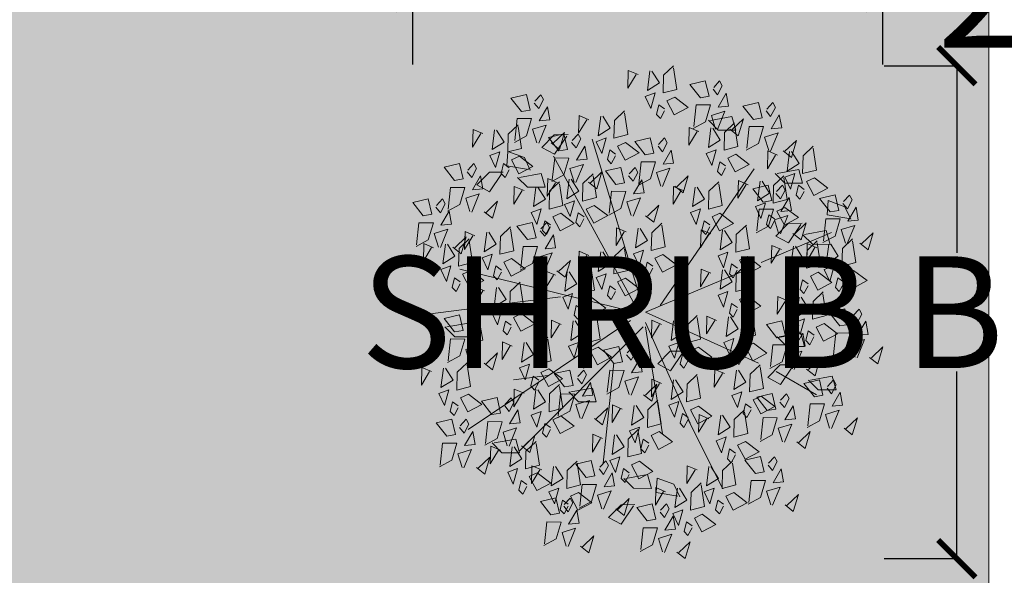
# Model space of a CAD drawing. Units: inches. Extents: x 1704 to 6393, y -157 to 1172.
# Tile 93 of 122: x 2667 to 2720, y 912 to 942. Entities that reach past the tile are written whole.
import ezdxf

# ---------------------------------------------------------------- set-up
doc = ezdxf.new("R2010")
doc.units = ezdxf.units.IN
doc.header["$MEASUREMENT"] = 0
for name, color, linetype, lineweight in [('A-ANNO-DIMS', 7, 'Continuous', 13), ('L-HRDS', 8, 'Continuous', 18), ('L-shrub', 74, 'Continuous', 18)]:
    doc.layers.add(name, color=color, linetype=linetype, lineweight=lineweight)
doc.layers.add('L-HRDS-PATT', color=9, linetype='Continuous', lineweight=13, true_color=0xc5c1ba)
doc.styles.get("Standard").update_dxf_attribs({"font": 'arial.ttf'})
doc.dimstyles.get("Standard").update_dxf_attribs({"dimtxt": 6, "dimasz": 2, "dimexe": 0.18, "dimexo": 0.0625, "dimgap": 0.09, "dimtad": 0, "dimtih": 1, "dimtoh": 1, "dimdec": 1, "dimzin": 0, "dimdsep": 46, "dimlunit": 3, "dimtxsty": 'Standard', "dimblk": 'ARCHTICK', "dimcen": 0.09, "dimadec": 0, "dimazin": 0, "dimtfac": 1, "dimtdec": 1, "dimtofl": 0, "dimtmove": 0, "dimatfit": 3, "dimfxl": 1, "dimtolj": 1, "dimtzin": 0, "dimarcsym": 0})

# ---------------------------------------------------------------- blocks, each defined once
blk = doc.blocks.new('flower shrub 2')
at = {"layer": 'L-shrub'}
for p, q in [((-106.2, 211.8), (-93, 218)), ((-112.6, 194.3), (-106.2, 211.8)), ((-93.7, 216.1), (-97.6, 193.3)), ((72, 198.6), (86.4, 202.7)), ((76, 175.8), (72, 198.6)), ((86.4, 202.7), (86.4, 184)), ((-97.6, 193.3), (-112.6, 194.3)), ((-81.1, 192.4), (-66.6, 196.5)), ((-77.1, 169.6), (-81.1, 192.4)), ((-66.6, 196.5), (-66.7, 177.9)), ((-66.7, 177.9), (-77.1, 167.5)), ((86.4, 184), (76, 173.7)), ((-145.2, 163.5), (-130.8, 167.5)), ((-130.8, 167.5), (-130.8, 148.9)), ((-88.7, 152.3), (-88.9, 166.9)), ((26.4, 165.5), (40.9, 169.6)), ((40.9, 169.6), (40.9, 151)), ((-141.2, 140.7), (-145.2, 163.5)), ((-87.4, 165.5), (-68.3, 152.5)), ((30.5, 142.8), (26.4, 165.5)), ((60.2, 144), (60.1, 158.6)), ((61.5, 157.2), (80.7, 144.2)), ((-130.8, 148.9), (-141.2, 138.6)), ((-75.4, 139.2), (-88.7, 152.3)), ((-68.3, 152.5), (-75.4, 139.2)), ((40.9, 151), (30.5, 140.7)), ((73.5, 131), (60.2, 144)), ((80.7, 144.2), (73.5, 131)), ((-201.1, 93.2), (-186.6, 97.3)), ((-197, 70.5), (-201.1, 93.2)), ((-186.6, 97.3), (-186.7, 78.7)), ((-186.7, 78.7), (-197.1, 68.4)), ((45.7, 28.3), (45.6, 42.9)), ((47.1, 41.5), (66.2, 28.5)), ((179.1, 14.6), (185.4, 32.1)), ((185.4, 32.1), (198.7, 38.3)), ((198, 36.3), (194.1, 13.5)), ((59, 15.3), (45.7, 28.3)), ((66.2, 28.5), (59, 15.3)), ((194.1, 13.5), (179.1, 14.6)), ((175.4, 4.4), (189.9, 8.5)), ((179.4, -18.4), (175.4, 4.4)), ((189.9, 8.5), (189.8, -10.1)), ((189.8, -10.1), (179.4, -20.5)), ((207.1, -23.3), (206.9, -8.7)), ((208.4, -10.1), (227.5, -23.1)), ((220.4, -36.4), (207.1, -23.3)), ((227.5, -23.1), (220.4, -36.4)), ((84.4, -53.5), (98.8, -49.4)), ((98.8, -49.4), (98.8, -68)), ((88.4, -76.2), (84.4, -53.5)), ((98.8, -68), (88.4, -78.3)), ((-181.8, -93.6), (-182, -78.9)), ((-180.5, -80.4), (-161.3, -93.4)), ((-168.5, -106.6), (-181.8, -93.6)), ((-161.3, -93.4), (-168.5, -106.6)), ((-141.1, -107.2), (-126.6, -103.1)), ((-126.6, -103.1), (-126.7, -121.7)), ((-137.1, -129.9), (-141.1, -107.2)), ((-157.9, -124.9), (-144.7, -118.7)), ((-145.4, -120.7), (-149.3, -143.5)), ((-126.7, -121.7), (-137.1, -132)), ((-164.3, -142.4), (-157.9, -124.9)), ((138.1, -134), (152.6, -130)), ((142.2, -156.8), (138.1, -134)), ((152.6, -130), (152.5, -148.6)), ((-149.3, -143.5), (-164.3, -142.4)), ((-142.5, -161.7), (-142.7, -147.1)), ((-141.2, -148.6), (-122, -161.6)), ((152.5, -148.6), (142.2, -158.9)), ((-129.2, -174.8), (-142.5, -161.7)), ((-122, -161.6), (-129.2, -174.8)), ((16.1, -183.6), (30.6, -179.5)), ((20.1, -206.4), (16.1, -183.6)), ((30.6, -179.5), (30.5, -198.1)), ((30.5, -198.1), (20.1, -208.5))]:
    blk.add_line(p, q, dxfattribs=at)
for points in [[(52.2, 237.8), (59.1, 246.6), (41.2, 251.8), (52.7, 239.8)], [(-67.8, 227.5), (-60.9, 236.2), (-78.8, 241.5), (-67.2, 229.5)], [(-39.3, 221.1), (-28.6, 235.3), (-20.7, 220.6), (-35.4, 212.7), (-39.3, 221.1)], [(10.2, 220.1), (16, 224.8), (6.6, 229.8), (1.5, 227), (8.2, 220.7)], [(29, 225.3), (28, 236.4), (14.3, 233.9), (29, 225.3)], [(52, 222.8), (37.8, 218.4), (33.4, 232.6), (52.6, 224.8)], [(-109.7, 209.7), (-104, 214.5), (-113.4, 219.4), (-118.5, 216.6), (-111.7, 210.3)], [(-90.9, 215), (-92, 226), (-105.6, 223.6), (-90.9, 215)], [(-68, 212.5), (-82.2, 208.1), (-86.6, 222.3), (-67.4, 214.4)], [(-70.4, 219.9), (-47.5, 223.4), (-43.8, 208.8), (-62.4, 209.3), (-72.5, 219.9)], [(49.5, 199.8), (26.5, 202.3), (26.7, 217.4), (44.5, 212.1), (51.5, 199.2)], [(126.6, 211), (133.5, 219.7), (115.7, 225), (127.2, 213)], [(-70.4, 189.5), (-93.4, 192), (-93.3, 207), (-75.4, 201.7), (-68.5, 188.9)], [(-27.2, 210.5), (-31.5, 204.4), (-21.2, 202), (-17, 206), (-25.1, 210.4)], [(19.2, 206.6), (5.2, 195.7), (1.3, 211.9), (17.6, 215.7), (19.2, 206.6)], [(103.5, 198.4), (102.5, 209.5), (88.8, 207.1), (103.5, 198.4)], [(-100.8, 196.3), (-114.8, 185.4), (-118.6, 201.6), (-102.4, 205.4), (-100.8, 196.3)], [(-47.6, 123.9), (-79, 197.9)], [(-66.9, 197.1), (-54.2, 205), (-46.3, 192.4), (-66.9, 195)], [(-44, 200.6), (-40.2, 190.1), (-27.6, 196), (-44, 200.6)], [(-37.3, 183.9), (-26.5, 198.1), (-18.6, 183.4), (-33.3, 175.6), (-37.3, 183.9)], [(16.5, 190.1), (27.3, 204.3), (35.1, 189.6), (20.4, 181.8), (16.5, 190.1)], [(84.7, 193.2), (90.4, 198), (81.1, 202.9), (75.9, 200.1), (82.7, 193.8)], [(126.5, 195.9), (112.2, 191.5), (107.8, 205.8), (127.1, 197.9)], [(-136.5, 179.8), (-125.8, 194), (-117.9, 179.3), (-132.6, 171.4), (-136.5, 179.8)], [(-14.5, 188.9), (8.3, 192.4), (12.1, 177.8), (-6.6, 178.4), (-16.6, 189)], [(93.7, 179.8), (79.6, 168.9), (75.8, 185.1), (92, 188.9), (93.7, 179.8)], [(124, 173), (101, 175.5), (101.1, 190.5), (119, 185.2), (126, 172.4)], [(-167.6, 178.6), (-144.8, 182.1), (-141, 167.5), (-159.6, 168), (-169.7, 178.6)], [(-68.3, 182.7), (-45.5, 186.2), (-41.7, 171.7), (-60.3, 172.2), (-70.4, 182.8)], [(-63.1, 182.5), (-67.5, 172.3), (-48.9, 171.8), (-63.2, 180.4)], [(28.7, 179.5), (24.4, 173.4), (34.6, 171), (38.9, 175.1), (30.7, 179.4)], [(64.6, 171.7), (71.5, 180.5), (53.6, 185.7), (65.1, 173.7)], [(66.9, 139.6), (91.6, 182.2)], [(-124.4, 169.1), (-128.7, 163.1), (-118.4, 160.7), (-114.2, 164.7), (-122.3, 169.1)], [(-78.2, 157.3), (-71.3, 166), (-89.1, 171.3), (-77.6, 159.2)], [(-64.8, 159.9), (-52.2, 167.8), (-44.2, 155.2), (-64.9, 157.8)], [(-25.1, 173.3), (-29.4, 167.2), (-19.1, 164.8), (-14.9, 168.9), (-23.1, 173.2)], [(-11, 166.1), (1.6, 174), (9.5, 161.4), (-11.1, 164)], [(11.8, 169.6), (15.7, 159.2), (28.3, 165), (11.8, 169.6)], [(41.4, 159.2), (40.4, 170.3), (26.7, 167.8), (41.4, 159.2)], [(64.4, 156.7), (50.2, 152.3), (45.8, 166.5), (65, 158.7)], [(141.1, 161.4), (148, 170.1), (130.1, 175.4), (141.7, 163.4)], [(-165, 146.9), (-158.1, 155.7), (-176, 160.9), (-164.5, 148.9)], [(-164.1, 155.7), (-151.5, 163.7), (-143.5, 151.1), (-164.1, 153.7)], [(-141.2, 159.3), (-137.4, 148.8), (-124.8, 154.7), (-141.2, 159.3)], [(-101.3, 144.7), (-102.3, 155.8), (-116, 153.4), (-101.3, 144.7)], [(-105.5, 148.8), (-94.8, 163), (-86.9, 148.3), (-101.6, 140.4), (-105.5, 148.8)], [(-41.9, 163.4), (-38.1, 153), (-25.5, 158.8), (-41.9, 163.4)], [(22.6, 154), (28.4, 158.7), (19, 163.6), (13.9, 160.9), (20.7, 154.6)], [(118, 148.8), (116.9, 159.9), (103.3, 157.5), (118, 148.8)], [(141, 146.3), (126.7, 141.9), (122.3, 156.2), (141.5, 148.3)], [(207.3, 149), (214.2, 157.7), (196.3, 163), (207.9, 151)], [(-188.2, 134.4), (-189.2, 145.5), (-202.9, 143), (-188.2, 134.4)], [(-136.6, 147.6), (-113.7, 151.1), (-110, 136.5), (-128.6, 137), (-138.7, 147.6)], [(-120.1, 139.5), (-114.4, 144.3), (-123.7, 149.2), (-128.8, 146.4), (-122.1, 140.1)], [(-78.3, 142.2), (-92.5, 137.8), (-97, 152), (-77.7, 144.2)], [(-61.1, 145.3), (-65.5, 135.1), (-46.9, 134.6), (-61.1, 143.2)], [(-7.3, 151.5), (-11.7, 141.3), (6.9, 140.8), (-7.3, 149.4)], [(31.6, 140.5), (17.6, 129.6), (13.8, 145.8), (30, 149.6), (31.6, 140.5)], [(61.9, 133.7), (39, 136.2), (39.1, 151.2), (56.9, 146), (63.9, 133.1)], [(99.2, 143.6), (104.9, 148.4), (95.6, 153.3), (90.4, 150.5), (97.2, 144.2)], [(184.2, 136.4), (183.1, 147.5), (169.5, 145.1), (184.2, 136.4)], [(-207, 129.2), (-201.2, 133.9), (-210.6, 138.9), (-215.7, 136.1), (-208.9, 129.8)], [(-165.2, 131.9), (-179.4, 127.5), (-183.8, 141.7), (-164.6, 133.9)], [(-160.3, 141.2), (-164.8, 131), (-146.1, 130.5), (-160.4, 139.1)], [(-111.1, 126.1), (-125.1, 115.1), (-129, 131.4), (-112.7, 135.2), (-111.1, 126.1)], [(-80.8, 119.3), (-103.8, 121.7), (-103.6, 136.8), (-85.8, 131.5), (-78.8, 118.7)], [(-93.4, 138.1), (-97.7, 132.1), (-87.4, 129.7), (-83.2, 133.7), (-91.3, 138.1)], [(108.1, 130.2), (94.1, 119.3), (90.3, 135.5), (106.5, 139.3), (108.1, 130.2)], [(93.1, 124), (103.8, 138.2), (111.7, 123.5), (97, 115.6), (93.1, 124)], [(138.5, 123.4), (115.5, 125.9), (115.6, 140.9), (133.5, 135.6), (140.5, 122.8)], [(165.4, 131.2), (171.1, 136), (161.8, 140.9), (156.6, 138.1), (163.4, 131.8)], [(207.2, 134), (192.9, 129.6), (188.5, 143.8), (207.7, 135.9)], [(-198, 115.7), (-212, 104.8), (-215.8, 121), (-199.6, 124.8), (-198, 115.7)], [(-167.7, 108.9), (-190.6, 111.4), (-190.5, 126.5), (-172.7, 121.2), (-165.7, 108.3)], [(-133.1, 124.8), (-120.4, 132.7), (-112.5, 120.1), (-133.1, 122.7)], [(-110.2, 128.3), (-106.3, 117.8), (-93.8, 123.7), (-110.2, 128.3)], [(37.2, 115.8), (47.9, 129.9), (55.8, 115.3), (41.1, 107.4), (37.2, 115.8)], [(62, 122.8), (84.8, 126.3), (88.6, 111.7), (70, 112.2), (59.9, 122.8)], [(174.3, 117.8), (160.3, 106.9), (156.5, 123.1), (172.7, 126.9), (174.3, 117.8)], [(204.7, 111), (181.7, 113.5), (181.8, 128.5), (199.7, 123.2), (206.7, 110.4)], [(-2.2, 17.9), (-145.9, 116.6)], [(-53.8, 109.6), (-43.1, 123.7), (-35.2, 109.1), (-49.9, 101.2), (-53.8, 109.6)], [(-12.4, 109.6), (-1.7, 123.7), (6.2, 109.1), (-8.5, 101.2), (-12.4, 109.6)], [(6.1, 114.5), (29, 118), (32.7, 103.5), (14.1, 104), (4.1, 114.6)], [(4.5, 2.2), (58.4, 121.1)], [(140.6, 107.5), (151.4, 121.7), (159.2, 107), (144.6, 99.1), (140.6, 107.5)], [(-187.8, 91.1), (-180.9, 99.9), (-198.7, 105.2), (-187.2, 93.1)], [(-161.4, 97.2), (-150.6, 111.3), (-142.8, 96.7), (-157.4, 88.8), (-161.4, 97.2)], [(-129.3, 110.2), (-133.7, 100), (-115.1, 99.5), (-129.4, 108.1)], [(-84.9, 108.3), (-62, 111.8), (-58.3, 97.3), (-76.9, 97.8), (-86.9, 108.4)], [(-43.5, 108.3), (-20.6, 111.8), (-16.9, 97.3), (-35.5, 97.8), (-45.6, 108.4)], [(4.5, 2.2), (-40.4, 109.9)], [(49.3, 105.1), (45, 99), (55.3, 96.7), (59.6, 100.7), (51.4, 105)], [(65.5, 100), (78.1, 107.9), (86.1, 95.3), (65.5, 97.9)], [(105.2, 113.4), (100.9, 107.3), (111.2, 104.9), (115.4, 108.9), (107.3, 113.3)], [(109.6, 106.3), (132.4, 109.8), (136.2, 95.2), (117.6, 95.7), (107.5, 106.3)], [(194.4, 95.1), (205.1, 109.3), (213, 94.6), (198.3, 86.7), (194.4, 95.1)], [(-192.4, 95.9), (-169.6, 99.4), (-165.8, 84.9), (-184.4, 85.4), (-194.5, 96)], [(-99.3, 80.6), (-88.6, 94.8), (-80.7, 80.1), (-95.4, 72.3), (-99.3, 80.6)], [(-81.3, 85.5), (-68.7, 93.4), (-60.8, 80.8), (-81.4, 83.4)], [(-41.7, 98.9), (-46, 92.8), (-35.7, 90.5), (-31.4, 94.5), (-39.6, 98.8)], [(-40, 85.5), (-27.4, 93.4), (-19.4, 80.8), (-40, 83.4)], [(-0.3, 98.9), (-4.6, 92.8), (5.7, 90.5), (9.9, 94.5), (1.8, 98.8)], [(9.7, 91.7), (22.3, 99.6), (30.2, 87), (9.6, 89.6)], [(32.5, 95.2), (36.4, 84.8), (49, 90.6), (32.5, 95.2)], [(88.4, 103.5), (92.2, 93), (104.8, 98.9), (88.4, 103.5)], [(152.8, 96.8), (148.5, 90.7), (158.7, 88.4), (163, 92.4), (154.8, 96.8)], [(163.3, 93.9), (186.2, 97.4), (189.9, 82.8), (171.3, 83.3), (161.3, 93.9)], [(-229.7, 73.4), (-224, 78.2), (-233.3, 83.1), (-238.5, 80.3), (-231.7, 74)], [(-210.9, 78.6), (-212, 89.7), (-225.6, 87.3), (-210.9, 78.6)], [(-187.9, 76.1), (-202.2, 71.7), (-206.6, 85.9), (-187.3, 78.1)], [(-149.2, 86.5), (-153.5, 80.4), (-143.3, 78.1), (-139, 82.1), (-147.2, 86.4)], [(-130.4, 79.4), (-107.5, 82.9), (-103.8, 68.4), (-122.4, 68.9), (-132.4, 79.5)], [(-58.5, 89), (-54.6, 78.6), (-42.1, 84.4), (-58.5, 89)], [(-17.1, 89), (-13.3, 78.6), (-0.7, 84.4), (-17.1, 89)], [(69.3, 85.4), (64.8, 75.2), (83.5, 74.7), (69.2, 83.3)], [(113.1, 83.4), (125.7, 91.4), (133.7, 78.7), (113, 81.4)], [(118.6, 47.7), (190.4, 83.6)], [(135.9, 87), (139.8, 76.5), (152.4, 82.4), (135.9, 87)], [(206.5, 84.4), (202.2, 78.4), (212.5, 76), (216.8, 80), (208.6, 84.4)], [(-188.9, 73.1), (-176.3, 81), (-168.3, 68.4), (-189, 71)], [(-166.1, 76.6), (-162.2, 66.2), (-149.6, 72), (-166.1, 76.6)], [(13.4, 77.1), (9, 66.9), (27.6, 66.4), (13.4, 75.1)], [(166.9, 71), (179.5, 79), (187.4, 66.3), (166.8, 69)], [(189.7, 74.6), (193.6, 64.1), (206.2, 70), (189.7, 74.6)], [(217.2, 62), (227.9, 76.2), (235.8, 61.5), (221.1, 53.7), (217.2, 62)], [(-220.7, 60), (-234.8, 49), (-238.6, 65.2), (-222.4, 69.1), (-220.7, 60)], [(-190.4, 53.1), (-213.4, 55.6), (-213.3, 70.7), (-195.4, 65.4), (-188.4, 52.6)], [(-126.9, 56.6), (-114.2, 64.5), (-106.3, 51.9), (-126.9, 54.5)], [(-87.2, 70), (-91.5, 63.9), (-81.2, 61.5), (-77, 65.6), (-85.1, 69.9)], [(-77.6, 70.9), (-82, 60.7), (-63.4, 60.2), (-77.7, 68.9)], [(-36.2, 70.9), (-40.6, 60.7), (-22, 60.2), (-36.3, 68.9)], [(41.4, 57.9), (52.1, 72.1), (60, 57.4), (45.3, 49.5), (41.4, 57.9)], [(103.4, 57.9), (114.1, 72.1), (122, 57.4), (107.3, 49.5), (103.4, 57.9)], [(116.8, 68.9), (112.4, 58.7), (131, 58.1), (116.8, 66.8)], [(186.1, 60.8), (209, 64.3), (212.7, 49.8), (194.1, 50.3), (184, 60.9)], [(-185.2, 58.5), (-189.6, 48.3), (-171, 47.8), (-185.2, 56.5)], [(-104, 60.1), (-100.1, 49.7), (-87.6, 55.5), (-104, 60.1)], [(10.3, 56.7), (33.1, 60.2), (36.9, 45.6), (18.3, 46.1), (8.2, 56.7)], [(72.3, 56.7), (95.2, 60.2), (98.9, 45.6), (80.3, 46.1), (70.3, 56.7)], [(170.6, 56.5), (166.2, 46.3), (184.8, 45.8), (170.6, 54.4)], [(-221.3, 33.1), (-210.6, 47.3), (-202.7, 32.6), (-217.4, 24.7), (-221.3, 33.1)], [(-127.8, 33.3), (-120.9, 42), (-138.8, 47.3), (-127.2, 35.3)], [(-123.1, 42), (-127.5, 31.8), (-108.9, 31.3), (-123.2, 39.9)], [(13.8, 33.9), (26.4, 41.8), (34.4, 29.2), (13.7, 31.8)], [(15.7, 2.2), (121.2, 49.3)], [(53.5, 47.2), (49.2, 41.2), (59.5, 38.8), (63.7, 42.8), (55.5, 47.2)], [(75.9, 33.9), (88.5, 41.8), (96.4, 29.2), (75.8, 31.8)], [(115.5, 47.2), (111.2, 41.2), (121.5, 38.8), (125.8, 42.8), (117.6, 47.2)], [(189.6, 38), (202.3, 45.9), (210.2, 33.3), (189.6, 35.9)], [(212.5, 41.5), (216.3, 31.1), (228.9, 36.9), (212.5, 41.5)], [(229.3, 51.4), (225, 45.3), (235.3, 43), (239.5, 47), (231.4, 51.3)], [(256.9, 35.4), (263.8, 44.1), (246, 49.4), (257.5, 37.3)], [(-252.4, 31.9), (-229.6, 35.4), (-225.8, 20.8), (-244.4, 21.3), (-254.5, 31.9)], [(-150.9, 20.8), (-152, 31.8), (-165.6, 29.4), (-150.9, 20.8)], [(-55.9, 20.7), (-45.1, 34.9), (-37.3, 20.2), (-52, 12.3), (-55.9, 20.7)], [(36.7, 37.4), (40.5, 26.9), (53.1, 32.8), (36.7, 37.4)], [(98.7, 37.4), (102.6, 26.9), (115.1, 32.8), (98.7, 37.4)], [(233.8, 22.8), (232.8, 33.9), (219.1, 31.5), (233.8, 22.8)], [(-209.2, 22.5), (-213.5, 16.4), (-203.2, 14), (-199, 18), (-207.2, 22.4)], [(-169.7, 15.5), (-164, 20.3), (-173.3, 25.2), (-178.5, 22.4), (-171.7, 16.1)], [(-127.9, 18.3), (-142.2, 13.9), (-146.6, 28.1), (-127.4, 20.2)], [(-86.9, 19.5), (-64.1, 23), (-60.3, 8.4), (-78.9, 8.9), (-89, 19.5)], [(130.3, 16.6), (141, 30.8), (148.9, 16.1), (134.2, 8.2), (130.3, 16.6)], [(193.4, 23.4), (189, 13.2), (207.6, 12.7), (193.3, 21.4)], [(215, 17.6), (220.7, 22.4), (211.4, 27.3), (206.3, 24.5), (213, 18.2)], [(256.8, 20.3), (242.6, 15.9), (238.1, 30.2), (257.4, 22.3)], [(-248.9, 9.1), (-236.3, 17), (-228.3, 4.4), (-249, 7)], [(-226, 12.6), (-222.2, 2.1), (-209.6, 8), (-226, 12.6)], [(-160.8, 2.1), (-174.8, -8.8), (-178.6, 7.4), (-162.4, 11.2), (-160.8, 2.1)], [(-130.4, -4.7), (-153.4, -2.2), (-153.3, 12.8), (-135.4, 7.5), (-128.4, -5.3)], [(-96.8, 2.3), (-89.9, 11), (-107.7, 16.3), (-96.2, 4.3)], [(17.5, 19.3), (13.1, 9.1), (31.7, 8.6), (17.5, 17.2)], [(20.2, 2.2), (132.5, 20.2)], [(79.6, 19.3), (75.2, 9.1), (93.8, 8.6), (79.5, 17.2)], [(91.5, 0.2), (98.4, 9), (80.5, 14.3), (92, 2.2)], [(99.2, 15.4), (122.1, 18.9), (125.8, 4.3), (107.2, 4.8), (97.2, 15.4)], [(224, 4.2), (210, -6.7), (206.1, 9.5), (222.4, 13.3), (224, 4.2)], [(254.3, -2.6), (231.3, -0.1), (231.5, 14.9), (249.3, 9.6), (256.3, -3.2)], [(0, 0), (-177.4, -53.8)], [(-119.9, -10.2), (-120.9, 0.8), (-134.6, -1.6), (-119.9, -10.2)], [(-83.4, -3.3), (-70.8, 4.6), (-62.9, -8), (-83.5, -5.4)], [(-60.6, 0.2), (-56.7, -10.3), (-44.1, -4.4), (-60.6, 0.2)], [(-43.7, 10.1), (-48, 4), (-37.8, 1.6), (-33.5, 5.7), (-41.7, 10)], [(20.2, 0), (150.4, -130.1)], [(102.7, -7.5), (115.4, 0.5), (123.3, -12.2), (102.7, -9.5)], [(142.4, 5.9), (138.1, -0.2), (148.4, -2.5), (152.7, 1.5), (144.5, 5.9)], [(161.3, -4.1), (172.1, 10.1), (179.9, -4.6), (165.2, -12.4), (161.3, -4.1)], [(-245.2, -5.5), (-249.6, -15.7), (-231, -16.2), (-245.2, -7.6)], [(-173.8, -18.5), (-163, -4.4), (-155.2, -19), (-169.9, -26.9), (-173.8, -18.5)], [(4.5, -4.5), (-159.4, -94.2)], [(-138.7, -15.4), (-133, -10.7), (-142.3, -5.8), (-147.4, -8.5), (-140.7, -14.9)], [(-96.9, -12.7), (-111.2, -17.1), (-115.6, -2.9), (-96.3, -10.7)], [(4.5, -9), (-40.4, -192.9)], [(-31, -18.5), (-20.3, -4.4), (-12.4, -19), (-27.1, -26.9), (-31, -18.5)], [(49.5, -17.5), (55.3, -12.7), (45.9, -7.8), (40.8, -10.6), (47.5, -16.9)], [(68.3, -12.3), (67.3, -1.2), (53.6, -3.6), (68.3, -12.3)], [(91.3, -14.8), (77.1, -19.2), (72.7, -5), (91.9, -12.8)], [(125.6, -4), (129.5, -14.4), (142, -8.5), (125.6, -4)], [(130.3, -5.3), (153.1, -1.8), (156.9, -16.3), (138.2, -15.8), (128.2, -5.2)], [(-204.8, -19.8), (-182, -16.2), (-178.2, -30.8), (-196.9, -30.3), (-206.9, -19.7)], [(-129.7, -28.9), (-143.8, -39.8), (-147.6, -23.6), (-131.4, -19.8), (-129.7, -28.9)], [(-99.4, -35.7), (-122.4, -33.2), (-122.3, -18.2), (-104.4, -23.4), (-97.4, -36.3)], [(-79.7, -17.9), (-84.1, -28.1), (-65.5, -28.6), (-79.7, -20)], [(-62.1, -19.8), (-39.3, -16.2), (-35.5, -30.8), (-54.1, -30.3), (-64.2, -19.7)], [(13.5, -13.5), (128, -183.9)], [(88.8, -37.8), (65.8, -35.3), (66, -20.2), (83.8, -25.5), (90.8, -38.3)], [(133.8, -28.1), (146.4, -20.2), (154.3, -32.8), (133.7, -30.2)], [(173.5, -14.7), (169.1, -20.8), (179.4, -23.2), (183.7, -19.1), (175.5, -14.8)], [(211.4, -28.7), (218.3, -19.9), (200.5, -14.7), (212, -26.7)], [(-161.6, -29.2), (-165.9, -35.3), (-155.7, -37.6), (-151.4, -33.6), (-159.6, -29.2)], [(-18.9, -29.2), (-23.2, -35.3), (-12.9, -37.6), (-8.7, -33.6), (-16.9, -29.2)], [(58.5, -30.9), (44.5, -41.9), (40.6, -25.7), (56.9, -21.8), (58.5, -30.9)], [(58, -30.8), (163.5, -42)], [(106.5, -22), (102.1, -32.2), (120.7, -32.8), (106.4, -24.1)], [(156.6, -24.6), (160.5, -35), (173.1, -29.2), (156.6, -24.6)], [(188.3, -41.2), (187.3, -30.1), (173.6, -32.6), (188.3, -41.2)], [(-201.3, -42.6), (-188.7, -34.7), (-180.8, -47.3), (-201.4, -44.7)], [(-178.5, -39.1), (-174.6, -49.5), (-162, -43.6), (-178.5, -39.1)], [(-107.6, -51.6), (-96.9, -37.4), (-89, -52.1), (-103.7, -60), (-107.6, -51.6)], [(-58.6, -42.6), (-46, -34.7), (-38, -47.3), (-58.7, -44.7)], [(-35.7, -39.1), (-31.9, -49.5), (-19.3, -43.6), (-35.7, -39.1)], [(-10.4, -53.7), (0.4, -39.5), (8.2, -54.2), (-6.4, -62), (-10.4, -53.7)], [(41.4, -47.5), (52.1, -33.3), (60, -48), (45.3, -55.8), (41.4, -47.5)], [(116.3, -51.4), (123.2, -42.7), (105.3, -37.4), (116.9, -49.4)], [(169.5, -46.4), (175.2, -41.7), (165.9, -36.7), (160.8, -39.5), (167.5, -45.8)], [(211.3, -43.7), (197, -48.1), (192.6, -33.9), (211.9, -41.7)], [(-131.9, -57.6), (-125, -48.9), (-142.9, -43.6), (-131.4, -55.6)], [(-138.7, -52.8), (-115.8, -49.3), (-112.1, -63.9), (-130.7, -63.4), (-140.7, -52.8)], [(-41.4, -54.9), (-18.6, -51.4), (-14.8, -65.9), (-33.4, -65.4), (-43.5, -54.8)], [(10.3, -48.7), (33.1, -45.2), (36.9, -59.7), (18.3, -59.2), (8.2, -48.6)], [(137.5, -42.7), (133.1, -52.9), (151.7, -53.4), (137.5, -44.8)], [(178.5, -59.9), (164.4, -70.8), (160.6, -54.6), (176.8, -50.8), (178.5, -59.9)], [(208.8, -66.7), (185.8, -64.2), (186, -49.1), (203.8, -54.4), (210.8, -67.3)], [(-197.6, -57.2), (-202, -67.4), (-183.4, -67.9), (-197.6, -59.2)], [(-155.1, -70.1), (-156.1, -59.1), (-169.8, -61.5), (-155.1, -70.1)], [(-54.9, -57.2), (-59.3, -67.4), (-40.7, -67.9), (-54.9, -59.2)], [(53.5, -58.1), (49.2, -64.2), (59.5, -66.5), (63.7, -62.5), (55.5, -58.2)], [(74.3, -69.2), (80.1, -64.4), (70.7, -59.5), (65.6, -62.3), (72.4, -68.6)], [(93.1, -63.9), (92.1, -52.9), (78.5, -55.3), (93.1, -63.9)], [(116.1, -66.4), (101.9, -70.8), (97.5, -56.6), (116.7, -64.5)], [(194.4, -68.1), (205.1, -53.9), (213, -68.6), (198.3, -76.5), (194.4, -68.1)], [(250.7, -65.9), (257.6, -57.1), (239.8, -51.9), (251.3, -63.9)], [(-173.9, -75.4), (-168.1, -70.6), (-177.5, -65.7), (-182.6, -68.5), (-175.9, -74.8)], [(-132.1, -72.6), (-146.3, -77), (-150.7, -62.8), (-131.5, -70.7)], [(-135.1, -75.6), (-122.5, -67.7), (-114.6, -80.3), (-135.2, -77.7)], [(-112.3, -72.1), (-108.4, -82.6), (-95.8, -76.7), (-112.3, -72.1)], [(-95.5, -62.2), (-99.8, -68.3), (-89.5, -70.7), (-85.2, -66.7), (-93.4, -62.3)], [(-37.9, -77.7), (-25.3, -69.8), (-17.3, -82.4), (-38, -79.8)], [(1.8, -64.3), (-2.5, -70.4), (7.7, -72.7), (12, -68.7), (3.8, -64.4)], [(13.8, -71.5), (26.4, -63.6), (34.4, -76.2), (13.7, -73.6)], [(36.7, -68), (40.5, -78.4), (53.1, -72.6), (36.7, -68)], [(113.7, -89.4), (90.7, -86.9), (90.8, -71.9), (108.7, -77.2), (115.6, -90)], [(163.3, -69.3), (186.2, -65.8), (189.9, -80.4), (171.3, -79.9), (161.3, -69.3)], [(227.6, -78.4), (226.6, -67.3), (212.9, -69.8), (227.6, -78.4)], [(250.6, -80.9), (236.3, -85.3), (231.9, -71.1), (251.2, -78.9)], [(-164.9, -88.8), (-178.9, -99.7), (-182.8, -83.5), (-166.5, -79.7), (-164.9, -88.8)], [(-134.6, -95.6), (-157.6, -93.1), (-157.4, -78.1), (-139.6, -83.4), (-132.6, -96.2)], [(-99.3, -86.7), (-88.6, -72.5), (-80.7, -87.2), (-95.4, -95.1), (-99.3, -86.7)], [(-38.9, -90.7), (-32, -81.9), (-49.8, -76.6), (-38.3, -88.7)], [(-15.1, -74.2), (-11.2, -84.6), (1.4, -78.8), (-15.1, -74.2)], [(83.3, -82.6), (69.3, -93.5), (65.5, -77.3), (81.7, -73.5), (83.3, -82.6)], [(113.7, -86.7), (124.5, -72.5), (132.4, -87.2), (117.7, -95.1), (113.7, -86.7)], [(208.8, -83.6), (214.5, -78.9), (205.2, -73.9), (200.1, -76.7), (206.8, -83)], [(206.5, -78.8), (202.2, -84.9), (212.5, -87.2), (216.8, -83.2), (208.6, -78.8)], [(-173.3, -96.9), (-166.4, -88.1), (-184.3, -82.8), (-172.7, -94.9)], [(-131.4, -90.2), (-135.8, -100.4), (-117.2, -100.9), (-131.4, -92.3)], [(-130.4, -87.9), (-107.5, -84.4), (-103.8, -99), (-122.4, -98.5), (-132.4, -87.9)], [(-62, -103.2), (-63, -92.1), (-76.7, -94.5), (-62, -103.2)], [(-34.2, -92.3), (-38.6, -102.5), (-20, -103), (-34.2, -94.3)], [(-4.9, -140.7), (-11.6, -86.9)], [(17.5, -86.1), (13.1, -96.3), (31.7, -96.8), (17.5, -88.1)], [(64.1, -99.1), (74.8, -84.9), (82.7, -99.6), (68, -107.5), (64.1, -99.1)], [(82.7, -87.9), (105.5, -84.4), (109.3, -99), (90.7, -98.5), (80.6, -87.9)], [(166.9, -92.2), (179.5, -84.2), (187.4, -96.9), (166.8, -94.2)], [(189.7, -88.7), (193.6, -99.1), (206.2, -93.2), (189.7, -88.7)], [(217.8, -97), (203.8, -108), (199.9, -91.8), (216.1, -87.9), (217.8, -97)], [(248.1, -103.9), (225.1, -101.4), (225.3, -86.3), (243.1, -91.6), (250.1, -104.5)], [(-196.4, -109.4), (-197.5, -98.3), (-211.1, -100.7), (-196.4, -109.4)], [(-173.4, -111.9), (-187.7, -116.3), (-192.1, -102.1), (-172.9, -109.9)], [(-126.9, -110.8), (-114.2, -102.8), (-106.3, -115.5), (-126.9, -112.8)], [(-87.2, -97.4), (-91.5, -103.5), (-81.2, -105.8), (-77, -101.8), (-85.1, -97.4)], [(-80.8, -108.4), (-75.1, -103.6), (-84.4, -98.7), (-89.5, -101.5), (-82.8, -107.8)], [(-39, -105.7), (-53.2, -110.1), (-57.7, -95.9), (-38.4, -103.7)], [(33, -100.3), (55.9, -96.8), (59.6, -111.4), (41, -110.9), (31, -100.3)], [(71.4, -100.3), (75.9, -136.2)], [(86.2, -110.8), (98.8, -102.8), (106.8, -115.5), (86.1, -112.8)], [(125.9, -97.4), (121.6, -103.5), (131.9, -105.8), (136.1, -101.8), (127.9, -97.4)], [(173.7, -111.5), (184.5, -97.3), (192.3, -112), (177.6, -119.9), (173.7, -111.5)], [(-215.2, -114.6), (-209.5, -109.8), (-218.8, -104.9), (-224, -107.7), (-217.2, -114)], [(-104, -107.2), (-100.1, -117.7), (-87.6, -111.8), (-104, -107.2)], [(-71.8, -121.8), (-85.8, -132.8), (-89.7, -116.6), (-73.4, -112.7), (-71.8, -121.8)], [(-41.5, -128.7), (-64.5, -126.2), (-64.3, -111.1), (-46.5, -116.4), (-39.5, -129.2)], [(76.2, -109.8), (71.9, -115.8), (82.2, -118.2), (86.5, -114.2), (78.3, -109.8)], [(109.1, -107.2), (112.9, -117.7), (125.5, -111.8), (109.1, -107.2)], [(145.2, -127.8), (152.1, -119.1), (134.3, -113.8), (145.8, -125.9)], [(142.7, -112.7), (165.5, -109.2), (169.3, -123.8), (150.7, -123.3), (140.6, -112.7)], [(170.6, -106.7), (166.2, -117), (184.8, -117.5), (170.6, -108.8)], [(-206.3, -128), (-220.3, -139), (-224.1, -122.8), (-207.9, -118.9), (-206.3, -128)], [(-175.9, -134.9), (-198.9, -132.4), (-198.8, -117.3), (-180.9, -122.6), (-173.9, -135.4)], [(-159.3, -130.1), (-148.6, -115.9), (-140.7, -130.6), (-155.4, -138.5), (-159.3, -130.1)], [(6.2, -128), (16.9, -113.8), (24.8, -128.5), (10.1, -136.4), (6.2, -128)], [(36.6, -123.2), (49.2, -115.2), (57.1, -127.8), (36.5, -125.2)], [(59.4, -119.6), (63.3, -130.1), (75.8, -124.2), (59.4, -119.6)], [(185.9, -122.2), (181.6, -128.2), (191.8, -130.6), (196.1, -126.6), (187.9, -122.2)], [(-190.4, -131.3), (-167.5, -127.8), (-163.8, -142.4), (-182.4, -141.9), (-192.4, -131.3)], [(-123.1, -125.3), (-127.5, -135.5), (-108.9, -136), (-123.2, -127.4)], [(-51.7, -138.4), (-41, -124.2), (-33.1, -138.9), (-47.8, -146.7), (-51.7, -138.4)], [(-24.9, -129.3), (-2, -125.7), (1.7, -140.3), (-16.9, -139.8), (-27, -129.2)], [(89.9, -125.3), (85.5, -135.5), (104.1, -136), (89.9, -127.4)], [(122.1, -140.4), (121.1, -129.3), (107.4, -131.7), (122.1, -140.4)], [(145.1, -142.9), (130.9, -147.3), (126.4, -133.1), (145.7, -140.9)], [(146.2, -135.6), (158.8, -127.6), (166.8, -140.2), (146.1, -137.6)], [(169, -132), (172.9, -142.5), (185.5, -136.6), (169, -132)], [(-147.2, -140.8), (-151.5, -146.8), (-141.2, -149.2), (-136.9, -145.2), (-145.1, -140.8)], [(-82.8, -139.6), (-59.9, -136.1), (-56.2, -150.6), (-74.8, -150.1), (-84.9, -139.5)], [(-21.4, -152.1), (-8.7, -144.2), (-0.8, -156.8), (-21.4, -154.1)], [(-4.5, -139), (6.7, -226.5)], [(18.3, -138.7), (14, -144.8), (24.3, -147.1), (28.5, -143.1), (20.4, -138.7)], [(40.3, -137.7), (35.9, -147.9), (54.5, -148.4), (40.2, -139.8)], [(103.3, -145.6), (109, -140.8), (99.7, -135.9), (94.6, -138.7), (101.3, -145)], [(-186.8, -154.1), (-174.2, -146.2), (-166.3, -158.8), (-186.9, -156.2)], [(-164, -150.6), (-160.1, -161.1), (-147.6, -155.2), (-164, -150.6)], [(-100.9, -167.1), (-94, -158.4), (-111.9, -153.1), (-100.3, -165.1)], [(-79.3, -162.4), (-66.7, -154.5), (-58.7, -167.1), (-79.3, -164.5)], [(-39.6, -149), (-43.9, -155.1), (-33.6, -157.4), (-29.4, -153.4), (-37.5, -149.1)], [(1.5, -148.6), (5.3, -159), (17.9, -153.1), (1.5, -148.6)], [(58.4, -167.1), (65.3, -158.4), (47.4, -153.1), (58.9, -165.1)], [(112.3, -159), (98.3, -170), (94.4, -153.7), (110.7, -149.9), (112.3, -159)], [(142.6, -165.8), (119.6, -163.4), (119.8, -148.3), (137.6, -153.6), (144.6, -166.4)], [(149.9, -150.1), (145.5, -160.3), (164.1, -160.8), (149.9, -152.2)], [(-56.4, -158.9), (-52.6, -169.3), (-40, -163.5), (-56.4, -158.9)], [(168, -175.4), (174.9, -166.6), (157, -161.3), (168.6, -173.4)], [(-183.1, -168.7), (-187.5, -178.9), (-168.9, -179.4), (-183.2, -170.8)], [(-142.8, -184.9), (-137.1, -180.1), (-146.4, -175.2), (-151.6, -178), (-144.8, -184.3)], [(-124, -179.6), (-125.1, -168.6), (-138.7, -171), (-124, -179.6)], [(-101.1, -182.1), (-115.3, -186.5), (-119.7, -172.3), (-100.5, -180.2)], [(-39.3, -181.7), (-28.6, -167.6), (-20.7, -182.2), (-35.4, -190.1), (-39.3, -181.7)], [(-17.6, -166.7), (-22, -176.9), (-3.4, -177.4), (-17.7, -168.7)], [(16.4, -184.9), (22.2, -180.1), (12.8, -175.2), (7.7, -178), (14.4, -184.3)], [(35.2, -179.6), (34.2, -168.6), (20.5, -171), (35.2, -179.6)], [(58.2, -182.1), (44, -186.5), (39.6, -172.3), (58.8, -180.2)], [(91, -183.8), (101.7, -169.6), (109.6, -184.3), (94.9, -192.2), (91, -183.8)], [(-75.5, -177), (-80, -187.2), (-61.3, -187.7), (-75.6, -179)], [(-63.7, -200.1), (-56.8, -191.4), (-74.6, -186.1), (-63.1, -198.2)], [(-70.4, -183), (-47.5, -179.5), (-43.8, -194), (-62.4, -193.5), (-72.5, -182.9)], [(59.9, -185), (82.8, -181.5), (86.5, -196.1), (67.9, -195.6), (57.9, -185)], [(126.1, -193.1), (131.8, -188.3), (122.5, -183.4), (117.3, -186.2), (124.1, -192.5)], [(144.9, -187.9), (143.8, -176.8), (130.2, -179.2), (144.9, -187.9)], [(167.9, -190.4), (153.6, -194.8), (149.2, -180.6), (168.4, -188.4)], [(-133.9, -198.3), (-147.9, -209.2), (-151.7, -193), (-135.5, -189.2), (-133.9, -198.3)], [(-103.5, -205.1), (-126.5, -202.6), (-126.4, -187.6), (-108.5, -192.8), (-101.6, -205.7)], [(-27.2, -192.4), (-31.5, -198.5), (-21.2, -200.8), (-17, -196.8), (-25.1, -192.5)], [(25.4, -198.3), (11.4, -209.2), (7.6, -193), (23.8, -189.2), (25.4, -198.3)], [(55.7, -205.1), (32.7, -202.6), (32.9, -187.6), (50.7, -192.8), (57.7, -205.7)], [(103.1, -194.5), (98.8, -200.6), (109.1, -202.9), (113.3, -198.9), (105.2, -194.5)], [(165.4, -213.4), (142.4, -210.9), (142.5, -195.8), (160.4, -201.1), (167.4, -214)], [(-86.8, -212.7), (-87.8, -201.6), (-101.5, -204), (-86.8, -212.7)], [(-63.8, -215.2), (-78.1, -219.6), (-82.5, -205.4), (-63.2, -213.2)], [(-66.9, -205.8), (-54.2, -197.9), (-46.3, -210.5), (-66.9, -207.9)], [(-44, -202.3), (-40.2, -212.7), (-27.6, -206.9), (-44, -202.3)], [(63.4, -207.9), (76.1, -199.9), (84, -212.6), (63.4, -209.9)], [(86.3, -204.3), (90.2, -214.8), (102.7, -208.9), (86.3, -204.3)], [(135, -206.5), (121, -217.5), (117.2, -201.3), (133.4, -197.4), (135, -206.5)], [(-105.6, -217.9), (-99.9, -213.1), (-109.2, -208.2), (-114.4, -211), (-107.6, -217.3)], [(-96.6, -231.3), (-110.7, -242.3), (-114.5, -226), (-98.3, -222.2), (-96.6, -231.3)], [(-66.3, -238.2), (-89.3, -235.7), (-89.2, -220.6), (-71.3, -225.9), (-64.3, -238.7)], [(-63.1, -220.4), (-67.5, -230.6), (-48.9, -231.1), (-63.2, -222.4)], [(67.2, -222.4), (62.8, -232.6), (81.4, -233.1), (67.1, -224.5)]]:
    blk.add_lwpolyline(points, dxfattribs=at)
blk = doc.blocks.new('_ArchTick')
at = {"color": 0, "linetype": 'ByBlock', "const_width": 0.15}
blk.add_lwpolyline([(-0.5, -0.5), (0.5, 0.5)], dxfattribs=at)
blk = doc.blocks.new('*D84')
at = {"layer": 'A-ANNO-DIMS', "color": 0, "lineweight": -2, "transparency": 16777216}
for p, q in [((2713.724, 939.698), (2717.812, 939.698)), ((2717.632, 939.698), (2717.632, 929.658)), ((2717.632, 913.234), (2717.632, 923.274)), ((2713.724, 913.234), (2717.812, 913.234))]:
    blk.add_line(p, q, dxfattribs=at)
at = {"layer": 'Defpoints', "color": 0, "lineweight": -3, "transparency": 16777216}
for p in [(2713.662, 939.698), (2713.662, 913.234), (2717.632, 913.234)]:
    blk.add_point(p, dxfattribs=at)
at = {"layer": 'A-ANNO-DIMS', "color": 0, "lineweight": -2, "transparency": 16777216, "xscale": 2, "yscale": 2, "zscale": 2}
for p, rotation in [((2717.632, 939.698), 90), ((2717.632, 913.234), 270)]:
    blk.add_blockref('_ArchTick', p, dxfattribs=dict(at, rotation=rotation))
at = {"layer": 'A-ANNO-DIMS', "color": 0, "transparency": 16777216, "insert": (2717.632, 926.466), "char_height": 6, "attachment_point": 5}
blk.add_mtext('\\A1;SHRUB B 26 TYP.', dxfattribs=at)
blk = doc.blocks.new('*D85')
at = {"layer": 'A-ANNO-DIMS', "color": 0, "lineweight": -2, "transparency": 16777216}
for p, q in [((2688.434, 939.761), (2688.434, 943.848)), ((2688.434, 943.668), (2713.662, 943.668)), ((2713.662, 939.761), (2713.662, 943.848)), ((2713.662, 943.668), (2715.662, 943.668))]:
    blk.add_line(p, q, dxfattribs=at)
at = {"layer": 'Defpoints', "color": 0, "lineweight": -3, "transparency": 16777216}
for p in [(2713.662, 943.668), (2688.434, 939.698), (2713.662, 939.698)]:
    blk.add_point(p, dxfattribs=at)
at = {"layer": 'A-ANNO-DIMS', "color": 0, "lineweight": -2, "transparency": 16777216, "xscale": 2, "yscale": 2, "zscale": 2, "rotation": 180}
blk.add_blockref('_ArchTick', (2688.434, 943.668), dxfattribs=at)
at = {"layer": 'A-ANNO-DIMS', "color": 0, "lineweight": -2, "transparency": 16777216, "xscale": 2, "yscale": 2, "zscale": 2}
blk.add_blockref('_ArchTick', (2713.662, 943.668), dxfattribs=at)
at = {"layer": 'A-ANNO-DIMS', "color": 0, "transparency": 16777216, "insert": (2730.406, 943.668), "char_height": 6, "attachment_point": 5}
blk.add_mtext('\\A1;25 TYP.', dxfattribs=at)
blk = doc.blocks.new('*D95')
at = {"layer": 'A-ANNO-DIMS', "color": 0, "lineweight": -2, "transparency": 16777216}
for p, q in [((2605.349, 895.275), (2605.349, 1105.287)), ((2605.349, 1105.107), (2657.907, 1105.107)), ((2723.349, 1105.107), (2670.791, 1105.107)), ((2723.349, 895.275), (2723.349, 1105.287))]:
    blk.add_line(p, q, dxfattribs=at)
at = {"layer": 'Defpoints', "color": 0, "lineweight": -3, "transparency": 16777216}
for p in [(2723.349, 1105.107), (2605.349, 895.213), (2723.349, 895.213)]:
    blk.add_point(p, dxfattribs=at)
at = {"layer": 'A-ANNO-DIMS', "color": 0, "lineweight": -2, "transparency": 16777216, "xscale": 2, "yscale": 2, "zscale": 2, "rotation": 180}
blk.add_blockref('_ArchTick', (2605.349, 1105.107), dxfattribs=at)
at = {"layer": 'A-ANNO-DIMS', "color": 0, "lineweight": -2, "transparency": 16777216, "xscale": 2, "yscale": 2, "zscale": 2}
blk.add_blockref('_ArchTick', (2723.349, 1105.107), dxfattribs=at)
at = {"layer": 'A-ANNO-DIMS', "color": 0, "transparency": 16777216, "insert": (2664.349, 1105.107), "char_height": 6, "attachment_point": 5}
blk.add_mtext('\\A1;118', dxfattribs=at)

msp = doc.modelspace()

# ---------------------------------------------------------------- hatches: boundary and pattern name
at = {"layer": 'L-HRDS-PATT', "transparency": 33554661}
h = msp.add_hatch(color=256, dxfattribs=at)
h.dxf.hatch_style = 1
h.paths.add_polyline_path([(2719.349, 1033.213), (2664.349, 1033.213), (2664.349, 895.213), (2719.349, 895.213)])
h.paths.add_polyline_path([(2719.349, 895.213), (2664.349, 895.213), (2605.349, 895.213), (2605.349, 872.213), (2719.349, 872.213)])
h.paths.add_polyline_path([(2719.349, 872.213), (2605.349, 872.213), (2605.349, 854.213), (2601.349, 854.213, -0.121066), (2618.034, 850.113), (2618.05, 850.14), (2619.349, 849.39), (2601.349, 818.213), (2605.349, 818.213), (2605.349, 794.213), (2605.349, 754.213), (2631.349, 754.213), (2631.349, 716.213), (2719.349, 716.213)])

# ---------------------------------------------------------------- linework, layer by layer
at = {"layer": 'L-HRDS'}
msp.add_line((2719.349, 5.658), (2719.349, 1033.213), dxfattribs=at)

# ---------------------------------------------------------------- block references
at = {"layer": 'L-shrub', "xscale": 0.0510581485411622, "yscale": 0.0510581485411622, "zscale": 0.0510581485411622, "rotation": 269.9999999999999}
msp.add_blockref('flower shrub 2', (2700.803, 926.705), dxfattribs=at)

# ---------------------------------------------------------------- dimensions: what is measured, and where the dimension line sits
at = {"layer": 'A-ANNO-DIMS'}
dim = msp.add_linear_dim(base=(2723.349, 1105.107), p1=(2605.349, 895.213), p2=(2723.349, 895.213), dimstyle='Standard', override={"dimdec": 0, "dimlfac": 1, "dimrnd": 0, "dimzin": 0, "dimdsep": 46, "dimlunit": 2}, dxfattribs=at)
dim.commit()
dim.dimension.update_dxf_attribs({"geometry": '*D95', "text_midpoint": (2664.349, 1105.107)})
dim = msp.add_linear_dim(base=(2713.662, 943.668), p1=(2688.434, 939.698), p2=(2713.662, 939.698), text='<> TYP.', dimstyle='Standard', override={"dimdec": 0, "dimlfac": 1, "dimrnd": 0, "dimzin": 0, "dimdsep": 46, "dimlunit": 2}, dxfattribs=at)
dim.commit()
dim.dimension.update_dxf_attribs({"geometry": '*D85', "text_midpoint": (2730.406, 943.668)})
dim = msp.add_linear_dim(base=(2717.632, 913.234), p1=(2713.662, 939.698), p2=(2713.662, 913.234), angle=270, text='SHRUB B <> TYP.', dimstyle='Standard', override={"dimdec": 0, "dimlfac": 1, "dimrnd": 0, "dimzin": 0, "dimdsep": 46, "dimlunit": 2}, dxfattribs=at)
dim.commit()
dim.dimension.update_dxf_attribs({"geometry": '*D84', "text_midpoint": (2717.632, 926.466)})

doc.saveas('drawing.dxf')
